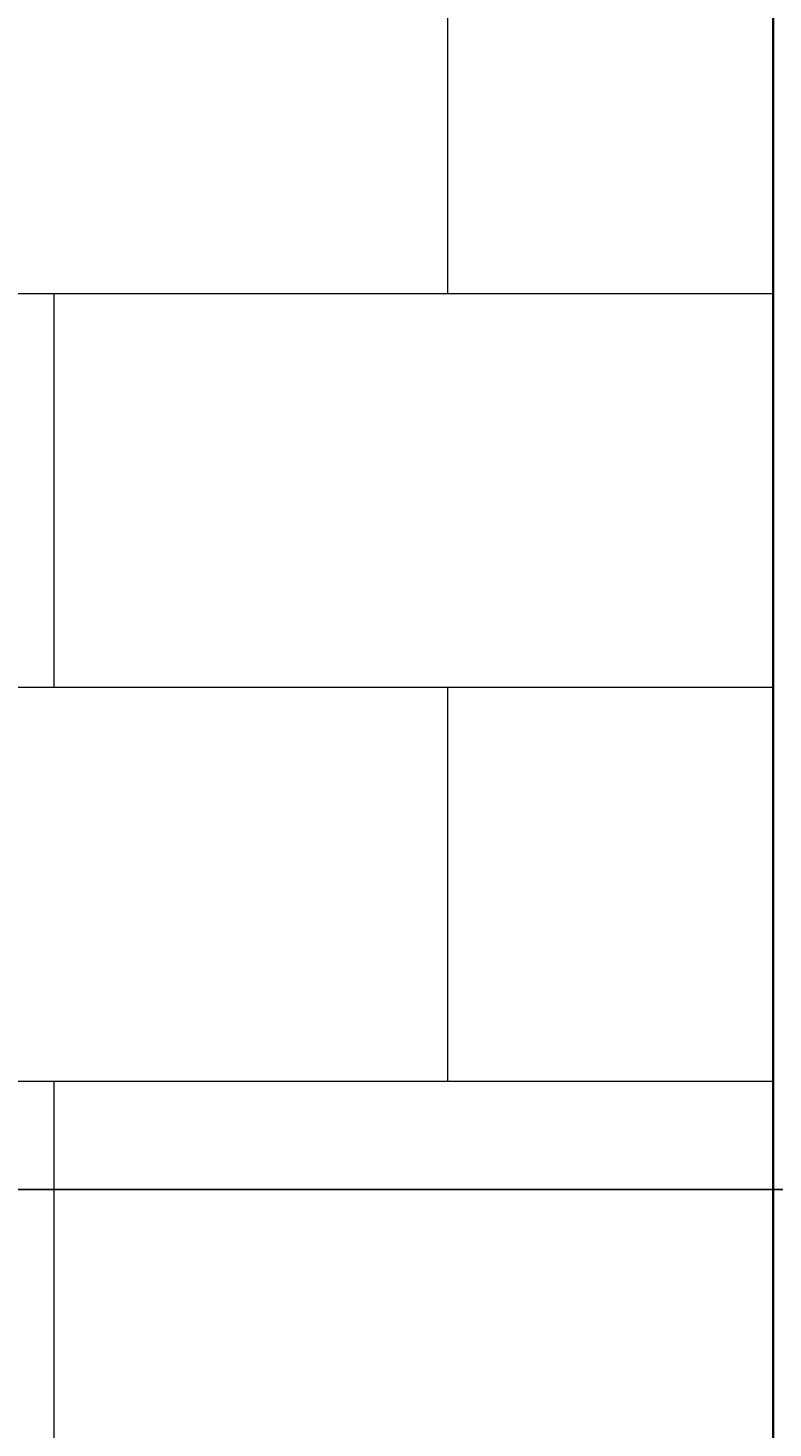
# Model space of a CAD drawing. Units: inches. Extents: x -26 to 776, y -22 to 650.
# Tile 25 of 62: x 358 to 426, y 292 to 420. Entities that reach past the tile are written whole.
import ezdxf

# ---------------------------------------------------------------- set-up
doc = ezdxf.new("R2010")
doc.units = ezdxf.units.IN
doc.header["$MEASUREMENT"] = 0
for name, color, linetype, lineweight in [('A-ANNO-DIMS', 2, 'Continuous', 18), ('A-WALL', 7, 'Continuous', 35), ('A-WALL-PATT', 8, 'Continuous', 13)]:
    doc.layers.add(name, color=color, linetype=linetype, lineweight=lineweight)
doc.styles.get("Standard").update_dxf_attribs({"font": 'arial.ttf'})
doc.dimstyles.get("Standard").update_dxf_attribs({"dimtxt": 0.5625, "dimasz": 0.18, "dimexe": 0.18, "dimexo": 0.0625, "dimgap": 0.09, "dimtad": 0, "dimtih": 1, "dimtoh": 1, "dimdec": 4, "dimzin": 0, "dimdsep": 46, "dimlunit": 4, "dimtxsty": 'Standard', "dimcen": 0.09, "dimadec": 0, "dimazin": 0, "dimtfac": 1, "dimtdec": 4, "dimtofl": 0, "dimtmove": 0, "dimatfit": 3, "dimfxl": 1, "dimtolj": 1, "dimtzin": 0, "dimarcsym": 0})

# ---------------------------------------------------------------- blocks, each defined once
blk = doc.blocks.new('*D28')
at = {"layer": 'A-ANNO-DIMS', "color": 0, "lineweight": -2, "transparency": 16777216}
for p, q in [((285.08, 314.12), (775.34, 314.12)), ((775.16, 313.94), (775.16, 243.14)), ((775.16, 171.6), (775.16, 242.4)), ((285.08, 171.42), (775.34, 171.42))]:
    blk.add_line(p, q, dxfattribs=at)
at = {"layer": 'A-ANNO-DIMS', "color": 0, "transparency": 16777216}
for points in [[(775.13, 313.94), (775.19, 313.94), (775.16, 314.12)], [(775.13, 171.6), (775.19, 171.6), (775.16, 171.42)]]:
    blk.add_solid(points, dxfattribs=at)
at = {"layer": 'Defpoints', "color": 0, "transparency": 16777216}
for p in [(285.02, 314.12), (775.16, 314.12), (285.02, 171.42)]:
    blk.add_point(p, dxfattribs=at)
at = {"layer": 'A-ANNO-DIMS', "color": 0, "transparency": 16777216, "insert": (775.16, 242.77), "char_height": 0.562, "attachment_point": 5}
blk.add_mtext('\\A1;142.7', dxfattribs=at)
blk = doc.blocks.new('*D39')
at = {"layer": 'A-ANNO-DIMS', "color": 0, "lineweight": -2, "transparency": 16777216}
for p, q in [((289.24, 15.54), (289.24, 649.86)), ((289.42, 649.68), (356.48, 649.68)), ((425.56, 649.68), (358.51, 649.68)), ((425.74, 15.54), (425.74, 649.86))]:
    blk.add_line(p, q, dxfattribs=at)
at = {"layer": 'A-ANNO-DIMS', "color": 0, "transparency": 16777216}
for points in [[(289.42, 649.71), (289.42, 649.65), (289.24, 649.68)], [(425.56, 649.71), (425.56, 649.65), (425.74, 649.68)]]:
    blk.add_solid(points, dxfattribs=at)
at = {"layer": 'Defpoints', "color": 0, "transparency": 16777216}
for p in [(425.74, 649.68), (289.24, 15.48), (425.74, 15.48)]:
    blk.add_point(p, dxfattribs=at)
at = {"layer": 'A-ANNO-DIMS', "color": 0, "transparency": 16777216, "insert": (357.49, 649.68), "char_height": 0.562, "attachment_point": 5}
blk.add_mtext('\\A1;136.5', dxfattribs=at)

msp = doc.modelspace()

# ---------------------------------------------------------------- hatches: boundary and pattern name
at = {"layer": 'A-WALL-PATT'}
h = msp.add_hatch(dxfattribs=at)
h.set_pattern_fill('AR-B816', color=256, scale=4.5)
h.paths.add_polyline_path([(425.7434, 448.2114), (289.2424, 496.9554), (289.2424, 458.1203), (289.2424, 291.1798), (289.2424, 20.7937), (425.7434, 20.7937), (425.7434, 283.2492)])

# ---------------------------------------------------------------- linework, layer by layer
at = {"layer": 'A-WALL'}
msp.add_line((425.7434, 283.2492), (425.7434, 455.4717), dxfattribs=at)

# ---------------------------------------------------------------- dimensions: what is measured, and where the dimension line sits
at = {"layer": 'A-ANNO-DIMS'}
dim = msp.add_linear_dim(base=(425.7434, 649.6763), p1=(289.2424, 15.4824), p2=(425.7434, 15.4824), dimstyle='Standard', override={"dimdec": 1, "dimlfac": 1, "dimrnd": 0, "dimzin": 0, "dimdsep": 46, "dimlunit": 2}, dxfattribs=at)
dim.commit()
dim.dimension.update_dxf_attribs({"geometry": '*D39', "text_midpoint": (357.4929, 649.6763)})
dim = msp.add_linear_dim(base=(775.1553, 314.119), p1=(285.0179, 171.4173), p2=(285.0179, 314.119), angle=90, dimstyle='Standard', override={"dimdec": 1, "dimlfac": 1, "dimrnd": 0, "dimzin": 0, "dimdsep": 46, "dimlunit": 2}, dxfattribs=at)
dim.commit()
dim.dimension.update_dxf_attribs({"geometry": '*D28', "text_midpoint": (775.1553, 242.7682)})

doc.saveas('drawing.dxf')
